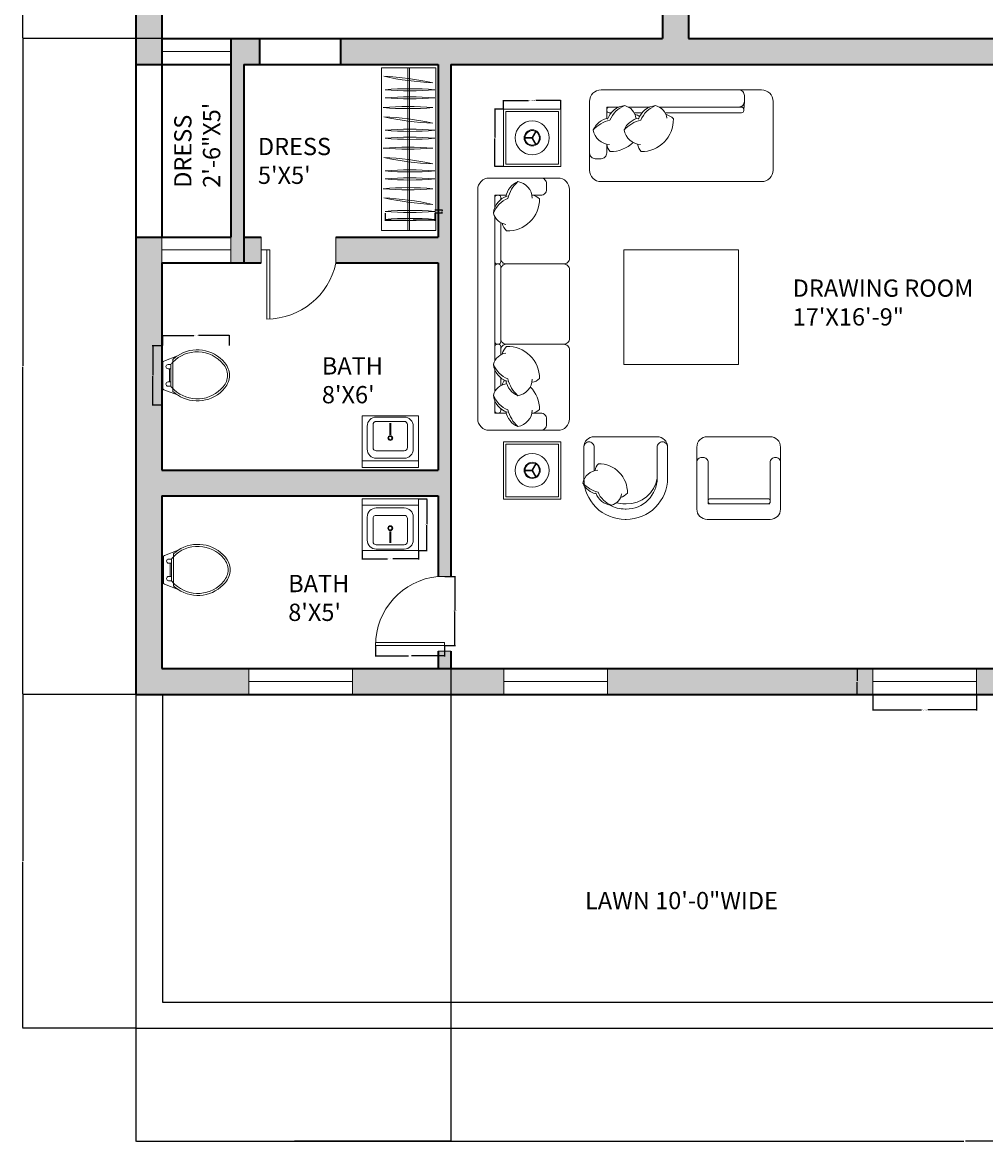
# Model space of a CAD drawing. Units: inches. Extents: x -9 to 646, y -802 to 47.
# Tile 1 of 17: x -9 to 326, y -802 to -412. Entities that reach past the tile are written whole.
import ezdxf

# ---------------------------------------------------------------- set-up
doc = ezdxf.new("R2010")
doc.units = ezdxf.units.IN
doc.header["$MEASUREMENT"] = 0
for name, color, linetype, lineweight in [('A-ANNO-DIMS', 2, 'Continuous', 18), ('A-AREA-IDEN', 7, 'Continuous', 18), ('A-DOOR', 4, 'Continuous', 18), ('A-FLOR-CASE', 8, 'Continuous', 18), ('A-FLOR-FIXT', 9, 'Continuous', 18), ('A-FURN', 8, 'Continuous', 15), ('A-GLAZ', 4, 'Continuous', 15), ('A-WALL', 7, 'Continuous', 35), ('A-WALL-PATT', 5, 'Continuous', 9), ('C-SITE', 7, 'Continuous', 25)]:
    doc.layers.add(name, color=color, linetype=linetype, lineweight=lineweight)
doc.styles.get("Standard").update_dxf_attribs({"font": 'arial.ttf'})
doc.dimstyles.get("Standard").update_dxf_attribs({"dimtxt": 0.18, "dimasz": 0.18, "dimexe": 0.18, "dimexo": 0.0625, "dimgap": 0.09, "dimtad": 0, "dimtih": 1, "dimtoh": 1, "dimdec": 0, "dimzin": 0, "dimdsep": 46, "dimlunit": 3, "dimtxsty": 'Standard', "dimcen": 0.09, "dimadec": 0, "dimazin": 0, "dimtfac": 1, "dimtdec": 0, "dimtofl": 0, "dimtmove": 0, "dimatfit": 3, "dimfxl": 1, "dimtolj": 1, "dimtzin": 0, "dimarcsym": 0})

# ---------------------------------------------------------------- blocks, each defined once
blk = doc.blocks.new('М14 600х655')
for p, q in [((-655, 600), (-655, 0)), ((-655, 600), (-655, 0)), ((-655, 0), (-655, 600)), ((0, 600), (-655, 600)), ((0, 525), (-655, 525)), ((0, 0), (0, 600)), ((-165, 494), (-490, 494)), ((-165, 408), (-490, 408)), ((-596, 388), (-596, 121)), ((-528, 370), (-528, 103)), ((-127, 103), (-127, 370)), ((-59, 121), (-59, 388)), ((-334, 87), (-334, 220)), ((-321, 87), (-321, 220)), ((-655, 0), (-655, 0)), ((-655, 0), (-655, 0)), ((-655, 0), (0, 0)), ((-655, 0), (0, 0)), ((-490, 65), (-165, 65)), ((-490, 15), (-165, 15))]:
    blk.add_line(p, q)
for radius in [27.6, 19.3]:
    blk.add_circle((-327, 259), radius)
for centre, radius, start, end in [((-490, 388), 106, 90, 180), ((-490, 370), 38.2, 90, 180), ((-165, 388), 106, 0, 90), ((-165, 370), 38.2, 0, 90), ((-490, 121), 106, 180, 270), ((-490, 103), 38.2, 180, 270), ((-165, 121), 106, 270, 0), ((-165, 103), 38.2, 270, 0)]:
    blk.add_arc(centre, radius, start, end)
blk = doc.blocks.new('WATER-CLOSET')
for p, q in [((3.52, 13.45), (3.52, 14.43)), ((3.52, 13.45), (3.52, 8.88)), ((3.52, 4.31), (3.52, 8.88)), ((3.52, 3.33), (3.52, 4.31))]:
    blk.add_line(p, q)
for points in [[(0, 8.88), (0, 13.32, -0.31031), (0.37, 13.86), (5.11, 15.69, -0.209071)], [(3.52, 13.45, -0.448546), (21.03, 12.81, -0.162618), (22.55, 8.88, -0.470877)], [(3.52, 14.43, -0.040937), (5.11, 15.69, -0.163732)], [(5.11, 15.69, -0.383919), (21.57, 13.25, -0.163732), (23.24, 8.88, -0.359733)], [(2.82, 12.65), (1.84, 12.65, 1), (1.84, 11.17), (2.35, 11.17)], [(2.82, 12.65, -0.022712), (3.52, 13.45, -0.162618)], [(2.82, 8.88), (2.82, 12.65, -0.476108)], [(0, 8.88), (0, 4.44, 0.31031), (0.37, 3.9), (5.11, 2.07, 0.209071)], [(2.82, 8.88), (2.82, 5.11, 0.022712)], [(3.99, 3.84, 0.431639), (21.03, 4.95, 0.162618), (22.55, 8.88, 0.470877)], [(5.11, 2.07, 0.383919), (21.57, 4.51, 0.163732), (23.24, 8.88, 0.359733)], [(2.82, 5.11), (1.84, 5.11, -1), (1.84, 6.59), (2.35, 6.59)], [(2.82, 5.11, 0.022712), (3.52, 4.31, 0.162618)], [(3.52, 4.31, 0.014165), (3.99, 3.84, 0.162618)], [(3.52, 3.33, 0.040937), (5.11, 2.07, 0.163732)]]:
    blk.add_lwpolyline(points, format="xyb")
for points in [[(2.35, 11.17), (2.35, 6.59)], [(2.35, 11.17), (2.82, 11.17)], [(2.35, 6.59), (2.82, 6.59)]]:
    blk.add_lwpolyline(points)
blk = doc.blocks.new('END-TABLE-SQUARE')
for p, q in [((9.86, 10.03), (11.26, 12.46)), ((10.07, 9.9), (11.48, 12.34)), ((9.96, 10.09), (7.15, 10.09)), ((9.96, 9.84), (7.15, 9.84)), ((9.86, 9.9), (11.26, 7.47)), ((10.07, 10.03), (11.48, 7.59))]:
    blk.add_line(p, q)
at = {"ltscale": 0.03}
blk.add_lwpolyline([(19.93, 19.93), (19.93, 0), (0, 0), (0, 19.93)], close=True, dxfattribs=at)
blk.add_lwpolyline([(19.13, 0.8), (19.13, 19.13), (0.8, 19.13), (0.8, 0.8)], close=True)
for radius in [5.88, 2.81, 2.52]:
    blk.add_circle((9.96, 9.97), radius)
blk = doc.blocks.new('CLOSET-GARMENT-SHORT')
for centre, start, end in [((8.63, -98.34), 85.0028, 94.9972), ((8.63, -98.34), 85.0028, 94.9972), ((8.63, 99.1), 265.0028, 274.9972), ((8.63, 99.1), 265.0028, 274.9972)]:
    blk.add_arc(centre, 99.09, start, end)
blk = doc.blocks.new('DOOR-LEAF-24-WALL9')
for p, q in [((0, 0), (0, 24)), ((1, 0), (1, 24)), ((0, 0), (1, 0))]:
    blk.add_line(p, q)
blk.add_arc((0, -0.52), 24.52, 11.8123, 90)
blk = doc.blocks.new('DOOR-LEAF-24-WALL4_5')
for p, q in [((0, 24), (24, 24)), ((0, 24), (0, 23)), ((0, 23), (24, 23))]:
    blk.add_line(p, q)
blk.add_arc((-0.11, 24), 24.12, 275.6311, 0)
blk = doc.blocks.new('GLAZING-36')
for p, q in [((0, 36), (0, 0)), ((4.5, 36), (4.5, 0)), ((9, 0), (9, 36))]:
    blk.add_line(p, q)
blk = doc.blocks.new('GLAZING-24')
for p, q in [((0, 9), (24, 9)), ((0, 4.5), (24, 4.5)), ((24, 0), (0, 0))]:
    blk.add_line(p, q)
blk = doc.blocks.new('*D19')
at = {"layer": 'A-ANNO-DIMS', "color": 0, "lineweight": -2, "transparency": 16777216}
for p, q in [((116.94, -478.74), (116.94, -481.44)), ((117.12, -481.26), (124.38, -481.26)), ((134.02, -481.26), (126.76, -481.26)), ((134.2, -478.74), (134.2, -481.44))]:
    blk.add_line(p, q, dxfattribs=at)
at = {"layer": 'A-ANNO-DIMS', "color": 0, "transparency": 16777216}
for points in [[(117.12, -481.23), (117.12, -481.29), (116.94, -481.26)], [(134.02, -481.23), (134.02, -481.29), (134.2, -481.26)]]:
    blk.add_solid(points, dxfattribs=at)
at = {"layer": 'Defpoints', "color": 0, "transparency": 16777216}
for p in [(116.94, -478.67), (134.2, -478.67), (134.2, -481.26)]:
    blk.add_point(p, dxfattribs=at)
at = {"layer": 'A-ANNO-DIMS', "color": 0, "transparency": 16777216, "insert": (125.57, -481.26), "char_height": 0.18, "attachment_point": 5}
blk.add_mtext('\\A1;GARMENT 17 TYP.', dxfattribs=at)
blk = doc.blocks.new('*D20')
at = {"layer": 'A-ANNO-DIMS', "color": 0, "lineweight": -2, "transparency": 16777216}
for p, q in [((134.26, -477.67), (136.97, -477.67)), ((136.79, -477.85), (136.79, -477.99)), ((136.79, -478.49), (136.79, -478.35)), ((134.26, -478.67), (136.97, -478.67))]:
    blk.add_line(p, q, dxfattribs=at)
at = {"layer": 'A-ANNO-DIMS', "color": 0, "transparency": 16777216}
for points in [[(136.76, -477.85), (136.82, -477.85), (136.79, -477.67)], [(136.76, -478.49), (136.82, -478.49), (136.79, -478.67)]]:
    blk.add_solid(points, dxfattribs=at)
at = {"layer": 'Defpoints', "color": 0, "transparency": 16777216}
for p in [(134.2, -477.67), (136.79, -477.67), (134.2, -478.67)]:
    blk.add_point(p, dxfattribs=at)
at = {"layer": 'A-ANNO-DIMS', "color": 0, "transparency": 16777216, "insert": (136.79, -478.17), "char_height": 0.18, "attachment_point": 5}
blk.add_mtext('\\A1;1 TYP.', dxfattribs=at)
blk = doc.blocks.new('*D23')
at = {"layer": 'A-ANNO-DIMS', "color": 0, "lineweight": -2, "transparency": 16777216}
for p, q in [((137.69, -605.07), (141.4, -605.07)), ((141.22, -605.25), (141.22, -616.89)), ((141.22, -628.89), (141.22, -617.25)), ((137.69, -629.07), (141.4, -629.07))]:
    blk.add_line(p, q, dxfattribs=at)
at = {"layer": 'A-ANNO-DIMS', "color": 0, "transparency": 16777216}
for points in [[(141.19, -605.25), (141.25, -605.25), (141.22, -605.07)], [(141.19, -628.89), (141.25, -628.89), (141.22, -629.07)]]:
    blk.add_solid(points, dxfattribs=at)
at = {"layer": 'Defpoints', "color": 0, "transparency": 16777216}
for p in [(137.62, -605.07), (137.62, -629.07), (141.22, -629.07)]:
    blk.add_point(p, dxfattribs=at)
at = {"layer": 'A-ANNO-DIMS', "color": 0, "transparency": 16777216, "insert": (141.22, -617.07), "char_height": 0.18, "attachment_point": 5}
blk.add_mtext('\\A1;DOOR 24 TYP.', dxfattribs=at)
blk = doc.blocks.new('*D24')
at = {"layer": 'A-ANNO-DIMS', "color": 0, "lineweight": -2, "transparency": 16777216}
for p, q in [((113.62, -629.13), (113.62, -632.85)), ((137.62, -629.13), (137.62, -632.85)), ((113.8, -632.67), (125.09, -632.67)), ((137.44, -632.67), (126.15, -632.67))]:
    blk.add_line(p, q, dxfattribs=at)
at = {"layer": 'A-ANNO-DIMS', "color": 0, "transparency": 16777216}
for points in [[(113.8, -632.64), (113.8, -632.7), (113.62, -632.67)], [(137.44, -632.64), (137.44, -632.7), (137.62, -632.67)]]:
    blk.add_solid(points, dxfattribs=at)
at = {"layer": 'Defpoints', "color": 0, "transparency": 16777216}
for p in [(113.62, -629.07), (137.62, -629.07), (113.62, -632.67)]:
    blk.add_point(p, dxfattribs=at)
at = {"layer": 'A-ANNO-DIMS', "color": 0, "transparency": 16777216, "insert": (125.62, -632.67), "char_height": 0.18, "attachment_point": 5}
blk.add_mtext('\\A1;24 TYP.', dxfattribs=at)
blk = doc.blocks.new('*D27')
at = {"layer": 'A-ANNO-DIMS', "color": 0, "lineweight": -2, "transparency": 16777216}
for p, q in [((286.47, -646.13), (286.47, -651.65)), ((322.47, -646.13), (322.47, -651.65)), ((286.65, -651.47), (303.35, -651.47)), ((322.29, -651.47), (305.59, -651.47))]:
    blk.add_line(p, q, dxfattribs=at)
at = {"layer": 'A-ANNO-DIMS', "color": 0, "transparency": 16777216}
for points in [[(286.65, -651.44), (286.65, -651.5), (286.47, -651.47)], [(322.29, -651.44), (322.29, -651.5), (322.47, -651.47)]]:
    blk.add_solid(points, dxfattribs=at)
at = {"layer": 'Defpoints', "color": 0, "transparency": 16777216}
for p in [(286.47, -646.07), (322.47, -646.07), (286.47, -651.47)]:
    blk.add_point(p, dxfattribs=at)
at = {"layer": 'A-ANNO-DIMS', "color": 0, "transparency": 16777216, "insert": (304.47, -651.47), "char_height": 0.18, "attachment_point": 5}
blk.add_mtext('\\A1;WINDOW 36 TYP.', dxfattribs=at)
blk = doc.blocks.new('*D28')
at = {"layer": 'A-ANNO-DIMS', "color": 0, "lineweight": -2, "transparency": 16777216}
for p, q in [((286.41, -637.07), (280.89, -637.07)), ((281.07, -637.25), (281.07, -641.39)), ((281.07, -645.89), (281.07, -641.75)), ((286.41, -646.07), (280.89, -646.07))]:
    blk.add_line(p, q, dxfattribs=at)
at = {"layer": 'A-ANNO-DIMS', "color": 0, "transparency": 16777216}
for points in [[(281.04, -637.25), (281.1, -637.25), (281.07, -637.07)], [(281.04, -645.89), (281.1, -645.89), (281.07, -646.07)]]:
    blk.add_solid(points, dxfattribs=at)
at = {"layer": 'Defpoints', "color": 0, "transparency": 16777216}
for p in [(281.07, -637.07), (286.47, -637.07), (286.47, -646.07)]:
    blk.add_point(p, dxfattribs=at)
at = {"layer": 'A-ANNO-DIMS', "color": 0, "transparency": 16777216, "insert": (281.07, -641.57), "char_height": 0.18, "attachment_point": 5}
blk.add_mtext('\\A1;9 TYP.', dxfattribs=at)
blk = doc.blocks.new('*D31')
at = {"layer": 'A-ANNO-DIMS', "color": 0, "lineweight": -2, "transparency": 16777216}
for p, q in [((108.99, -596.07), (108.99, -599.12)), ((109.17, -598.94), (117.83, -598.94)), ((128.36, -598.94), (119.7, -598.94)), ((128.54, -596.07), (128.54, -599.12))]:
    blk.add_line(p, q, dxfattribs=at)
at = {"layer": 'A-ANNO-DIMS', "color": 0, "transparency": 16777216}
for points in [[(109.17, -598.91), (109.17, -598.97), (108.99, -598.94)], [(128.36, -598.91), (128.36, -598.97), (128.54, -598.94)]]:
    blk.add_solid(points, dxfattribs=at)
at = {"layer": 'Defpoints', "color": 0, "transparency": 16777216}
for p in [(108.99, -596), (128.54, -596), (128.54, -598.94)]:
    blk.add_point(p, dxfattribs=at)
at = {"layer": 'A-ANNO-DIMS', "color": 0, "transparency": 16777216, "insert": (118.76, -598.94), "char_height": 0.18, "attachment_point": 5}
blk.add_mtext('\\A1;BASIN 20 TYP.', dxfattribs=at)
blk = doc.blocks.new('*D32')
at = {"layer": 'A-ANNO-DIMS', "color": 0, "lineweight": -2, "transparency": 16777216}
for p, q in [((128.6, -578.1), (131.65, -578.1)), ((131.47, -578.28), (131.47, -586.87)), ((131.47, -595.82), (131.47, -587.23)), ((128.6, -596), (131.65, -596))]:
    blk.add_line(p, q, dxfattribs=at)
at = {"layer": 'A-ANNO-DIMS', "color": 0, "transparency": 16777216}
for points in [[(131.44, -578.28), (131.5, -578.28), (131.47, -578.1)], [(131.44, -595.82), (131.5, -595.82), (131.47, -596)]]:
    blk.add_solid(points, dxfattribs=at)
at = {"layer": 'Defpoints', "color": 0, "transparency": 16777216}
for p in [(128.54, -578.1), (131.47, -578.1), (128.54, -596)]:
    blk.add_point(p, dxfattribs=at)
at = {"layer": 'A-ANNO-DIMS', "color": 0, "transparency": 16777216, "insert": (131.47, -587.05), "char_height": 0.18, "attachment_point": 5}
blk.add_mtext('\\A1;18 TYP.', dxfattribs=at)
blk = doc.blocks.new('*D33')
at = {"layer": 'A-ANNO-DIMS', "color": 0, "lineweight": -2, "transparency": 16777216}
for p, q in [((39.69, -524.77), (39.69, -521.17)), ((62.93, -524.77), (62.93, -521.17)), ((39.87, -521.35), (50.54, -521.35)), ((62.75, -521.35), (52.09, -521.35))]:
    blk.add_line(p, q, dxfattribs=at)
at = {"layer": 'A-ANNO-DIMS', "color": 0, "transparency": 16777216}
for points in [[(39.87, -521.32), (39.87, -521.38), (39.69, -521.35)], [(62.75, -521.32), (62.75, -521.38), (62.93, -521.35)]]:
    blk.add_solid(points, dxfattribs=at)
at = {"layer": 'Defpoints', "color": 0, "transparency": 16777216}
for p in [(39.69, -524.84), (62.93, -521.35), (62.93, -524.84)]:
    blk.add_point(p, dxfattribs=at)
at = {"layer": 'A-ANNO-DIMS', "color": 0, "transparency": 16777216, "insert": (51.31, -521.35), "char_height": 0.18, "attachment_point": 5}
blk.add_mtext('\\A1;WC 23 TYP.', dxfattribs=at)
blk = doc.blocks.new('*D34')
at = {"layer": 'A-ANNO-DIMS', "color": 0, "lineweight": -2, "transparency": 16777216}
for p, q in [((39.63, -524.84), (36.02, -524.84)), ((36.2, -525.02), (36.2, -534.98)), ((36.2, -545.31), (36.2, -535.34)), ((39.63, -545.49), (36.02, -545.49))]:
    blk.add_line(p, q, dxfattribs=at)
at = {"layer": 'A-ANNO-DIMS', "color": 0, "transparency": 16777216}
for points in [[(36.17, -525.02), (36.23, -525.02), (36.2, -524.84)], [(36.17, -545.31), (36.23, -545.31), (36.2, -545.49)]]:
    blk.add_solid(points, dxfattribs=at)
at = {"layer": 'Defpoints', "color": 0, "transparency": 16777216}
for p in [(36.2, -524.84), (39.69, -524.84), (39.69, -545.49)]:
    blk.add_point(p, dxfattribs=at)
at = {"layer": 'A-ANNO-DIMS', "color": 0, "transparency": 16777216, "insert": (36.2, -535.16), "char_height": 0.18, "attachment_point": 5}
blk.add_mtext('\\A1;21 TYP.', dxfattribs=at)
blk = doc.blocks.new('*D39')
at = {"layer": 'A-ANNO-DIMS', "color": 0, "lineweight": -2, "transparency": 16777216}
for p, q in [((158.14, -442.59), (158.14, -439.48)), ((178.07, -442.59), (178.07, -439.48)), ((158.32, -439.66), (166.81, -439.66)), ((177.89, -439.66), (169.39, -439.66))]:
    blk.add_line(p, q, dxfattribs=at)
at = {"layer": 'A-ANNO-DIMS', "color": 0, "transparency": 16777216}
for points in [[(158.32, -439.63), (158.32, -439.69), (158.14, -439.66)], [(177.89, -439.63), (177.89, -439.69), (178.07, -439.66)]]:
    blk.add_solid(points, dxfattribs=at)
at = {"layer": 'Defpoints', "color": 0, "transparency": 16777216}
for p in [(158.14, -442.65), (178.07, -439.66), (178.07, -442.65)]:
    blk.add_point(p, dxfattribs=at)
at = {"layer": 'A-ANNO-DIMS', "color": 0, "transparency": 16777216, "insert": (168.1, -439.66), "char_height": 0.18, "attachment_point": 5}
blk.add_mtext('\\A1;SIDE TABLE 20 TYP.', dxfattribs=at)
blk = doc.blocks.new('*D40')
at = {"layer": 'A-ANNO-DIMS', "color": 0, "lineweight": -2, "transparency": 16777216}
for p, q in [((158.08, -442.65), (154.97, -442.65)), ((155.15, -442.83), (155.15, -452.43)), ((155.15, -462.4), (155.15, -452.8)), ((158.08, -462.58), (154.97, -462.58))]:
    blk.add_line(p, q, dxfattribs=at)
at = {"layer": 'A-ANNO-DIMS', "color": 0, "transparency": 16777216}
for points in [[(155.12, -442.83), (155.18, -442.83), (155.15, -442.65)], [(155.12, -462.4), (155.18, -462.4), (155.15, -462.58)]]:
    blk.add_solid(points, dxfattribs=at)
at = {"layer": 'Defpoints', "color": 0, "transparency": 16777216}
for p in [(155.15, -442.65), (158.14, -442.65), (158.14, -462.58)]:
    blk.add_point(p, dxfattribs=at)
at = {"layer": 'A-ANNO-DIMS', "color": 0, "transparency": 16777216, "insert": (155.15, -452.61), "char_height": 0.18, "attachment_point": 5}
blk.add_mtext('\\A1;20 TYP.', dxfattribs=at)
blk = doc.blocks.new('*D49')
at = {"layer": 'A-ANNO-DIMS', "color": 0, "lineweight": -2, "transparency": 16777216}
for p, q in [((30.37, -762.13), (30.37, -801.5)), ((606.37, -762.13), (606.37, -801.5)), ((30.55, -801.32), (318.08, -801.32)), ((606.19, -801.32), (318.66, -801.32))]:
    blk.add_line(p, q, dxfattribs=at)
at = {"layer": 'A-ANNO-DIMS', "color": 0, "transparency": 16777216}
for points in [[(30.55, -801.29), (30.55, -801.35), (30.37, -801.32)], [(606.19, -801.29), (606.19, -801.35), (606.37, -801.32)]]:
    blk.add_solid(points, dxfattribs=at)
at = {"layer": 'Defpoints', "color": 0, "transparency": 16777216}
for p in [(30.37, -762.07), (606.37, -762.07), (606.37, -801.32)]:
    blk.add_point(p, dxfattribs=at)
at = {"layer": 'A-ANNO-DIMS', "color": 0, "transparency": 16777216, "insert": (318.37, -801.32), "char_height": 0.18, "attachment_point": 5}
blk.add_mtext('\\A1;576', dxfattribs=at)
blk = doc.blocks.new('*D55')
at = {"layer": 'A-ANNO-DIMS', "color": 0, "lineweight": -2, "transparency": 16777216}
for p, q in [((39.31, -253.07), (-9.06, -253.07)), ((-8.88, -253.25), (-8.88, -335.39)), ((-8.88, -417.89), (-8.88, -335.75)), ((39.31, -418.07), (-9.06, -418.07))]:
    blk.add_line(p, q, dxfattribs=at)
at = {"layer": 'A-ANNO-DIMS', "color": 0, "transparency": 16777216}
for points in [[(-8.91, -253.25), (-8.85, -253.25), (-8.88, -253.07)], [(-8.91, -417.89), (-8.85, -417.89), (-8.88, -418.07)]]:
    blk.add_solid(points, dxfattribs=at)
at = {"layer": 'Defpoints', "color": 0, "transparency": 16777216}
for p in [(39.37, -253.07), (-8.88, -418.07), (39.37, -418.07)]:
    blk.add_point(p, dxfattribs=at)
at = {"layer": 'A-ANNO-DIMS', "color": 0, "transparency": 16777216, "insert": (-8.88, -335.57), "char_height": 0.18, "attachment_point": 5}
blk.add_mtext('\\A1;165', dxfattribs=at)
blk = doc.blocks.new('*D56')
at = {"layer": 'A-ANNO-DIMS', "color": 0, "lineweight": -2, "transparency": 16777216}
for p, q in [((213.31, -418.07), (-9.06, -418.07)), ((-8.88, -418.25), (-8.88, -531.89)), ((-8.88, -645.89), (-8.88, -532.25)), ((30.31, -646.07), (-9.06, -646.07))]:
    blk.add_line(p, q, dxfattribs=at)
at = {"layer": 'A-ANNO-DIMS', "color": 0, "transparency": 16777216}
for points in [[(-8.91, -418.25), (-8.85, -418.25), (-8.88, -418.07)], [(-8.91, -645.89), (-8.85, -645.89), (-8.88, -646.07)]]:
    blk.add_solid(points, dxfattribs=at)
at = {"layer": 'Defpoints', "color": 0, "transparency": 16777216}
for p in [(213.37, -418.07), (-8.88, -646.07), (30.37, -646.07)]:
    blk.add_point(p, dxfattribs=at)
at = {"layer": 'A-ANNO-DIMS', "color": 0, "transparency": 16777216, "insert": (-8.88, -532.07), "char_height": 0.18, "attachment_point": 5}
blk.add_mtext('\\A1;228', dxfattribs=at)
blk = doc.blocks.new('*D57')
at = {"layer": 'A-ANNO-DIMS', "color": 0, "lineweight": -2, "transparency": 16777216}
for p, q in [((30.31, -646.07), (-9.06, -646.07)), ((-8.88, -646.25), (-8.88, -703.89)), ((-8.88, -761.89), (-8.88, -704.25)), ((30.31, -762.07), (-9.06, -762.07))]:
    blk.add_line(p, q, dxfattribs=at)
at = {"layer": 'A-ANNO-DIMS', "color": 0, "transparency": 16777216}
for points in [[(-8.91, -646.25), (-8.85, -646.25), (-8.88, -646.07)], [(-8.91, -761.89), (-8.85, -761.89), (-8.88, -762.07)]]:
    blk.add_solid(points, dxfattribs=at)
at = {"layer": 'Defpoints', "color": 0, "transparency": 16777216}
for p in [(30.37, -646.07), (-8.88, -762.07), (30.37, -762.07)]:
    blk.add_point(p, dxfattribs=at)
at = {"layer": 'A-ANNO-DIMS', "color": 0, "transparency": 16777216, "insert": (-8.88, -704.07), "char_height": 0.18, "attachment_point": 5}
blk.add_mtext('\\A1;116', dxfattribs=at)
blk = doc.blocks.new('*D58')
at = {"layer": 'A-ANNO-DIMS', "color": 0, "lineweight": -2, "transparency": 16777216}
for p, q in [((139.87, -637.13), (139.87, -801.5)), ((30.37, -646.13), (30.37, -801.5)), ((30.55, -801.32), (84.74, -801.32)), ((139.69, -801.32), (85.51, -801.32))]:
    blk.add_line(p, q, dxfattribs=at)
at = {"layer": 'A-ANNO-DIMS', "color": 0, "transparency": 16777216}
for points in [[(30.55, -801.29), (30.55, -801.35), (30.37, -801.32)], [(139.69, -801.29), (139.69, -801.35), (139.87, -801.32)]]:
    blk.add_solid(points, dxfattribs=at)
at = {"layer": 'Defpoints', "color": 0, "transparency": 16777216}
for p in [(139.87, -637.07), (30.37, -646.07), (139.87, -801.32)]:
    blk.add_point(p, dxfattribs=at)
at = {"layer": 'A-ANNO-DIMS', "color": 0, "transparency": 16777216, "insert": (85.12, -801.32), "char_height": 0.18, "attachment_point": 5}
blk.add_mtext('\\A1;109.5', dxfattribs=at)

msp = doc.modelspace()

# ---------------------------------------------------------------- hatches: boundary and pattern name
at = {"layer": 'A-WALL-PATT'}
h = msp.add_hatch(color=256, dxfattribs=at)
h.dxf.hatch_style = 1
h.paths.add_polyline_path([(73.4, -418.07), (63.37, -418.07), (63.37, -487.07), (63.35, -496.07), (67.87, -496.07), (67.87, -427.07), (73.4, -427.07)])
h.paths.add_polyline_path([(73.87, -487.07), (67.87, -487.07), (67.87, -496.07), (73.87, -496.07)])
h.paths.add_polyline_path([(39.37, -496.07), (39.35, -496.07), (39.35, -487.07), (30.37, -487.07), (30.37, -646.07), (69.62, -646.07), (69.62, -637.07), (39.37, -637.07)])
h.paths.add_polyline_path([(158.27, -637.07), (105.62, -637.07), (105.62, -646.07), (158.27, -646.07)])
h.paths.add_polyline_path([(286.47, -637.07), (194.27, -637.07), (194.27, -646.07), (286.47, -646.07)])
h.paths.add_polyline_path([(357.37, -552.07), (352.87, -552.07), (348.37, -552.07), (348.37, -637.07), (322.47, -637.07), (322.47, -646.07), (357.37, -646.07)])
h.paths.add_polyline_path([(357.37, -459.07), (352.87, -459.07), (348.37, -459.07), (348.37, -526.07), (357.37, -526.07), (357.37, -520.07), (363.37, -520.07), (363.37, -511.07), (357.37, -511.07)], flags=17)
h.paths.add_polyline_path([(39.37, -262.07), (213.37, -262.07), (213.37, -268.07), (222.37, -268.07), (222.37, -247.07), (213.37, -247.07), (213.37, -253.07), (39.37, -253.07), (39.37, -1.07), (222.37, -1.07), (222.37, 7.93), (30.37, 7.93), (30.37, -427.07), (39.36, -427.07), (39.36, -418.07)])
h.paths.add_polyline_path([(570.37, -149.32), (561.37, -149.32), (561.37, -161.07), (433.37, -161.07), (433.37, -165.57), (433.37, -170.07), (438.37, -170.07), (438.37, -176.07), (447.37, -176.07), (447.37, -170.07), (561.37, -170.07), (561.37, -229.57), (570.37, -229.57)])
h.paths.add_polyline_path([(570.37, -289.57), (561.37, -289.57), (561.37, -349.07), (479.37, -349.07), (479.37, -353.57), (479.37, -358.07), (561.37, -358.07), (561.37, -418.07), (447.37, -418.07), (447.37, -358.07), (453.37, -358.07), (453.37, -349.07), (447.37, -349.07), (447.37, -202.07), (442.87, -202.07), (438.37, -202.07), (438.37, -427.07), (561.37, -427.07), (561.37, -451.07), (570.37, -451.07)])
h.paths.add_polyline_path([(570.37, -496.07), (570.37, -487.07), (561.37, -487.07), (561.37, -511.07), (411.37, -511.07), (411.37, -515.57), (411.37, -520.07), (570.37, -520.07)])
h = msp.add_hatch(color=256, dxfattribs=at)
h.dxf.hatch_style = 1
h.paths.add_polyline_path([(363.37, -418.07), (222.37, -418.07), (222.37, -294.07), (217.87, -294.07), (213.37, -294.07), (213.37, -418.07), (101.62, -418.07), (101.62, -427.07), (135.37, -427.07), (135.37, -487.07), (99.87, -487.07), (99.87, -491.57), (99.87, -496.07), (135.37, -496.07), (135.37, -568.07), (39.37, -568.07), (39.37, -496.07), (39.35, -496.07), (39.35, -487.07), (30.37, -487.07), (30.37, -646.07), (69.62, -646.07), (69.62, -637.07), (39.37, -637.07), (39.37, -577.07), (135.37, -577.07), (135.37, -605.07), (137.62, -605.07), (139.87, -605.07), (139.87, -427.07), (348.37, -427.07), (348.37, -433.07), (357.37, -433.07), (357.37, -427.07), (363.37, -427.07)])
h = msp.add_hatch(color=256, dxfattribs=at)
h.dxf.hatch_style = 1
h.paths.add_polyline_path([(139.87, -631.07), (135.37, -631.07), (135.37, -637.07), (139.87, -637.07)])

# ---------------------------------------------------------------- linework, layer by layer
at = {"layer": 'A-DOOR'}
for p, q in [((73.87, -496.07), (73.87, -487.07)), ((99.87, -491.57), (99.87, -487.07)), ((73.87, -491.57), (75.87, -491.57)), ((99.87, -491.57), (99.87, -496.07)), ((137.62, -605.07), (135.37, -605.07)), ((137.62, -605.07), (139.87, -605.07)), ((137.62, -631.07), (137.62, -629.07)), ((139.87, -631.07), (135.37, -631.07))]:
    msp.add_line(p, q, dxfattribs=at)
at = {"layer": 'A-FLOR-CASE'}
for p, q in [((115.77, -428.3), (115.77, -484.79)), ((115.77, -428.3), (134.61, -428.3)), ((115.77, -428.3), (115.77, -484.79)), ((115.77, -428.3), (134.61, -428.3)), ((124.88, -428.3), (124.88, -484.79)), ((124.88, -428.3), (124.88, -484.79)), ((125.5, -428.3), (125.5, -484.79)), ((125.5, -428.3), (125.5, -484.79)), ((134.61, -428.3), (134.61, -484.79)), ((134.61, -428.3), (134.61, -484.79)), ((115.77, -484.79), (134.61, -484.79))]:
    msp.add_line(p, q, dxfattribs=at)
at = {"layer": 'A-FURN'}
msp.add_line((241.83, -439.92), (241.64, -442.91), dxfattribs=at)
at = {"layer": 'A-FURN', "ltscale": 0.03}
for points in [[(251.8, -463.83, -0.414214), (247.81, -467.81), (247.81, -467.81, 0.317837), (247.81, -467.81, -0.414214), (247.81, -467.81), (247.81, -467.81, 1.186185), (247.81, -467.81, -0.414214), (247.81, -467.81), (192.02, -467.81, -0.414214), (188.03, -463.83), (188.03, -439.92, -0.414214), (192.02, -435.93), (247.81, -435.93, -0.414214), (251.8, -439.92)], [(177.07, -466.56, -0.414214), (181.06, -470.55), (181.06, -494.46, -0.414214), (179.06, -496.45, -0.414214), (181.06, -498.45), (181.06, -522.36, -0.414214), (179.06, -524.35, -0.414214), (181.06, -526.34), (181.06, -550.26, -0.414214), (177.07, -554.24), (153.16, -554.24, -0.414214), (149.17, -550.26), (149.17, -470.55, -0.414214), (153.16, -466.56)], [(250.81, -585.22), (250.81, -585.22, 0.414214), (254.4, -581.63), (254.4, -560.07, 0.414214), (250.81, -556.48), (250.81, -556.48), (228.89, -556.48, 0.414214), (225.3, -560.07), (225.3, -581.63, 0.414214), (228.89, -585.22)]]:
    msp.add_lwpolyline(points, format="xyb", close=True, dxfattribs=at)
at = {"layer": 'A-FURN'}
for points in [[(236.75, -441.91), (239.84, -441.91, 0.414214), (241.83, -439.92), (241.83, -437.92, 0.414214), (239.84, -435.93)], [(189.3, -449.86, -0.14773), (195.12, -446.44, -0.213343), (200.26, -441.41, -0.178662)], [(195.53, -443.9), (194.81, -443.9, -0.414214), (194.01, -443.11), (194.01, -442.71, -0.414214), (194.81, -441.91)], [(198.2, -441.91), (194.01, -441.91), (194.01, -445.83, -0.414214)], [(194.32, -446.16, -0.306663), (200.26, -441.41, -0.30633), (204.14, -445.75, 0.872847)], [(194.81, -441.91), (198.2, -441.91, -0.414214)], [(200.03, -449.86, -0.14773), (205.86, -446.44, -0.213343), (211, -441.41, -0.178662)], [(201.52, -441.91), (208.94, -441.91, -0.414214)], [(205.05, -446.16, -0.306663), (211, -441.41, -0.30633), (214.88, -445.75, 0.872847)], [(212.25, -441.91), (240.84, -441.91, -0.414214), (241.64, -442.71), (241.64, -443.11, -0.414214), (240.84, -443.9), (214.26, -443.9, -0.414214)], [(195.01, -454.88, -0.356772), (189.3, -449.86, -0.249542), (194.47, -445.72, 9.61688)], [(205.74, -454.88, -0.356772), (200.03, -449.86, -0.249542), (205.21, -445.72, 9.61688)], [(206.26, -443.9), (203.52, -443.9, -0.414214)], [(205.44, -445.19, 0.071865), (203.77, -444.41, -7.115464)], [(204.74, -454.76, 0.165541), (205.97, -457.4, 0.425989), (217.16, -445.98, 0.121523), (214.51, -444.41, -7.115464)], [(194.01, -454.76), (194.01, -457.85, -0.414214), (192.02, -459.84), (190.02, -459.84, -0.414214), (188.03, -457.85)], [(194, -454.76, 0.165541), (195.24, -457.4, 0.200231), (203.15, -454.19, 0.121523)], [(171.09, -466.56, -0.414214), (173.09, -468.56), (173.09, -470.55, -0.414214), (171.09, -472.54), (168.01, -472.54)], [(163.1, -467.83, 0.14773), (159.68, -473.66, 0.213343), (154.66, -478.79)], [(168.13, -473.54, 0.356772), (163.1, -467.83, 0.249542), (158.96, -473)], [(159.41, -472.85, 0.306663), (154.66, -478.79, 0.30633), (158.99, -482.68)], [(157.14, -474.06), (157.14, -473.34, 0.414214), (156.35, -472.54), (155.95, -472.54, 0.414214), (155.15, -473.34)], [(155.15, -473.34), (155.15, -476.73, 0.412535)], [(168, -472.54, -0.165541), (170.64, -473.77, -0.425989), (159.22, -484.96, -0.121523), (157.65, -482.3)], [(155.15, -480.05), (155.15, -495.66, 0.414214), (155.95, -496.45), (156.35, -496.45, 0.414214), (157.14, -495.66), (157.14, -482.05, 0.412652)], [(157.14, -494.46, 0.414214), (159.14, -496.45), (179.06, -496.45, 0.415249)], [(157.14, -498.45, -0.414214), (159.14, -496.45)], [(155.15, -530.02), (155.15, -525.15, -0.414214), (155.95, -524.35), (156.35, -524.35, -0.414214), (157.14, -525.15), (157.14, -528.01, -0.126313)], [(157.14, -522.36, 0.414214), (159.14, -524.35)], [(157.14, -526.34, -0.414214), (159.14, -524.35), (179.06, -524.35, -0.41732)], [(168, -537.53, 0.165541), (170.64, -536.3, 0.425989), (159.22, -525.11, 0.121523), (157.65, -527.77)], [(159.41, -537.22, -0.306663), (154.66, -531.28, -0.30633), (158.99, -527.39)], [(163.1, -542.24, -0.14773), (159.68, -536.41, -0.213343), (154.66, -531.28)], [(155.15, -540.76), (155.15, -533.34, -0.414747)], [(157.14, -536.01), (157.14, -538.75, -0.414599)], [(158.43, -536.83, 0.071865), (157.65, -538.5)], [(168.13, -536.53, -0.356772), (163.1, -542.24, -0.249542), (158.96, -537.06)], [(159.41, -547.95, -0.306663), (154.66, -542.01, -0.30633), (158.99, -538.13)], [(168, -548.27, 0.165541), (170.64, -547.03, 0.200231), (167.43, -539.12)], [(163.1, -552.97, -0.14773), (159.68, -547.15, -0.213343), (154.66, -542.01)], [(155.15, -544.07), (155.15, -548.26), (159.07, -548.26, -0.414352)], [(155.15, -547.47), (155.15, -544.07, -0.414469)], [(157.14, -546.74), (157.14, -547.47, -0.414214), (156.35, -548.26), (155.95, -548.26, -0.414214), (155.15, -547.47)], [(168.13, -547.26, -0.356772), (163.1, -552.97, -0.249542), (158.96, -547.8)], [(168.01, -548.26), (171.09, -548.26, -0.414214), (173.09, -550.26), (173.09, -552.25, -0.414214), (171.09, -554.24)], [(189.62, -568.33), (189.62, -560.07, 0.414214), (187.83, -558.27), (187.83, -558.27, 0.414214), (186.03, -560.07)], [(211.54, -570.85), (211.54, -560.07, -0.414214), (213.34, -558.27), (213.34, -558.27, -0.414214), (215.14, -560.07)], [(225.3, -565.46, -0.414214), (227.09, -563.66), (227.45, -563.66, -0.414214), (229.25, -565.46), (229.25, -568.24)], [(250.81, -578.75), (250.81, -565.46, -0.414214), (252.61, -563.66), (252.61, -563.66, -0.414214), (254.4, -565.46)], [(189.98, -568.24, -0.165541), (191.09, -565.87, -0.425989), (201.18, -576.16, -0.121523), (198.79, -577.58, 7.115464)], [(190.89, -568.13, 0.356772), (185.74, -572.66, 0.249542), (190.4, -576.39, -9.61688)], [(211.54, -570.85, -0.372719), (200.76, -579.83), (200.58, -579.83)], [(211.54, -570.85, -0.414214), (200.76, -581.63), (200.58, -581.63)], [(185.74, -572.66, 0.14773), (190.99, -575.75, 0.213343), (195.62, -580.28, 0.178662)], [(190.26, -576, 0.306663), (195.62, -580.28, 0.30633), (199.12, -576.37, -0.872847)], [(197.34, -579.45, 0.072384), (200.41, -579.83), (200.58, -579.83)], [(237.83, -578.04), (229.97, -578.04, 0.414214), (229.25, -578.75), (229.25, -579.11, 0.414214), (229.97, -579.83)], [(236.02, -579.83), (250.09, -579.83, 0.414214), (250.81, -579.11), (250.81, -578.75, 0.414214), (250.09, -578.04), (237.83, -578.04, 0.414214)], [(195.05, -580.21, 0.130591), (200.41, -581.63), (200.58, -581.63)], [(229.97, -579.83), (236.02, -579.83, 0.414214)]]:
    msp.add_lwpolyline(points, format="xyb", dxfattribs=at)
for points in [[(208.94, -441.91), (201.52, -441.91)], [(236.75, -441.91), (212.25, -441.91)], [(159.07, -472.54), (155.15, -472.54), (155.15, -476.73)], [(155.15, -480.05), (155.15, -530.02)], [(155.15, -533.34), (155.15, -540.76)], [(229.25, -568.24), (229.25, -579.83), (236.02, -579.83)], [(236.02, -579.83), (250.63, -579.83)]]:
    msp.add_lwpolyline(points, dxfattribs=at)
at = {"layer": 'A-FURN', "ltscale": 0.03}
msp.add_lwpolyline([(239.84, -531.33), (239.84, -491.47), (199.99, -491.47), (199.99, -531.33)], close=True, dxfattribs=at)
at = {"layer": 'A-FURN'}
msp.add_lwpolyline([(155.15, -523.55), (155.15, -497.25, -0.414214), (155.95, -496.45), (156.35, -496.45, -0.414214), (157.14, -497.25), (157.14, -523.55, -0.414214), (156.35, -524.35), (155.95, -524.35, -0.414214)], format="xyb", close=True, dxfattribs=at)
at = {"layer": 'A-FURN', "ltscale": 0.03}
msp.add_lwpolyline([(200.58, -556.48), (211.54, -556.48, -0.414214), (215.14, -560.07), (215.14, -570.85, -0.414214), (200.76, -585.22), (200.58, -585.22), (200.41, -585.22, -0.414214), (186.03, -570.85), (186.03, -560.07, -0.414214), (189.62, -556.48), (200.58, -556.48)], format="xyb", dxfattribs=at)
at = {"layer": 'A-GLAZ'}
for p, q in [((39.36, -427.07), (39.36, -418.07)), ((63.36, -418.07), (63.36, -427.07)), ((63.35, -487.07), (39.35, -487.07)), ((39.35, -487.07), (39.35, -496.07)), ((63.35, -496.07), (63.35, -487.07)), ((39.35, -491.57), (63.35, -491.57)), ((39.35, -496.07), (63.35, -496.07)), ((69.62, -637.07), (69.62, -646.07)), ((105.62, -646.07), (105.62, -637.07)), ((158.27, -637.07), (158.27, -646.07)), ((194.27, -646.07), (194.27, -637.07)), ((286.47, -637.07), (286.47, -646.07)), ((322.47, -646.07), (322.47, -637.07))]:
    msp.add_line(p, q, dxfattribs=at)
at = {"layer": 'A-WALL'}
for p, q in [((30.37, 7.93), (30.37, -646.07)), ((39.37, -262.07), (39.37, -487.07)), ((213.37, -294.07), (213.37, -418.07)), ((222.37, -294.07), (222.37, -418.07)), ((39.37, -418.07), (213.37, -418.07)), ((63.37, -418.07), (63.37, -487.07)), ((73.4, -427.07), (73.4, -418.07)), ((101.62, -427.07), (101.62, -418.07)), ((222.37, -418.07), (438.37, -418.07)), ((30.37, -427.07), (63.37, -427.07)), ((67.87, -427.07), (67.87, -496.07)), ((67.87, -427.07), (135.37, -427.07)), ((135.37, -427.07), (135.37, -487.07)), ((139.87, -427.07), (348.37, -427.07)), ((139.87, -427.07), (139.87, -605.07)), ((30.37, -487.07), (63.37, -487.07)), ((67.87, -487.07), (73.87, -487.07)), ((99.87, -487.07), (135.37, -487.07)), ((39.37, -496.07), (73.87, -496.07)), ((39.37, -496.07), (39.37, -568.07)), ((99.87, -496.07), (135.37, -496.07)), ((135.37, -496.07), (135.37, -568.07)), ((39.37, -568.07), (135.37, -568.07)), ((39.37, -577.07), (135.37, -577.07)), ((39.37, -577.07), (39.37, -637.07)), ((135.37, -577.07), (135.37, -605.07)), ((135.37, -631.07), (135.37, -637.07)), ((139.87, -631.07), (139.87, -637.07)), ((39.37, -637.07), (348.37, -637.07)), ((213.37, -637.07), (222.37, -637.07)), ((213.37, -637.07), (222.37, -637.07)), ((30.37, -646.07), (357.37, -646.07))]:
    msp.add_line(p, q, dxfattribs=at)
at = {"layer": 'C-SITE'}
for p, q in [((30.37, -646.07), (30.37, -762.07)), ((39.59, -646.07), (39.59, -753.07)), ((39.59, -753.07), (348.37, -753.07)), ((30.37, -762.07), (606.37, -762.07))]:
    msp.add_line(p, q, dxfattribs=at)

# ---------------------------------------------------------------- block references
at = {"layer": 'A-DOOR', "extrusion": (0, 0, -1), "zscale": -1, "rotation": 180}
msp.add_blockref('DOOR-LEAF-24-WALL9', (-75.87, -491.57), dxfattribs=at)
at = {"layer": 'A-DOOR', "rotation": 180}
msp.add_blockref('DOOR-LEAF-24-WALL4_5', (137.63, -605.07), dxfattribs=at)
at = {"layer": 'A-FLOR-CASE'}
for p, rotation in [((116.43, -431.58), 352.5051423896663), ((134.2, -435.51), 180), ((133.59, -441.69), 180), ((116.43, -445.65), 352.5051423895279), ((134.2, -449.59), 180), ((133.64, -461.28), 172.505142389491), ((134.2, -466.51), 180), ((133.64, -475.35), 172.505142389491), ((134.2, -480.58), 180)]:
    msp.add_blockref('CLOSET-GARMENT-SHORT', p, dxfattribs=dict(at, rotation=rotation))
for p in [(116.94, -439.06), (116.94, -453.14), (116.33, -456.58), (116.94, -464.48), (116.33, -470.66), (116.94, -478.55)]:
    msp.add_blockref('CLOSET-GARMENT-SHORT', p, dxfattribs=at)
at = {"layer": 'A-FLOR-FIXT'}
for p in [(39.69, -544.04), (39.91, -611.65)]:
    msp.add_blockref('WATER-CLOSET', p, dxfattribs=at)
at = {"layer": 'A-FLOR-FIXT', "xscale": -0.0298457359050645, "yscale": 0.0298457359050645, "zscale": 0.0298457359050645, "rotation": 180}
msp.add_blockref('М14 600х655', (128.54, -549.22), dxfattribs=at)
at = {"layer": 'A-FLOR-FIXT', "xscale": 0.0298457359050645, "yscale": 0.0298457359050645, "zscale": 0.0298457359050645}
msp.add_blockref('М14 600х655', (128.54, -596), dxfattribs=at)
at = {"layer": 'A-FURN'}
msp.add_blockref('END-TABLE-SQUARE', (158.14, -462.58), dxfattribs=at)
at = {"layer": 'A-FURN', "extrusion": (0, 0, -1), "zscale": -1, "rotation": 180}
msp.add_blockref('END-TABLE-SQUARE', (-158.14, -558.22), dxfattribs=at)
at = {"layer": 'A-GLAZ'}
msp.add_blockref('GLAZING-24', (39.36, -427.07), dxfattribs=at)
for p, rotation in [((105.62, -646.07), 90.00000000000036), ((194.27, -646.07), 90.00000000000003), ((322.47, -646.07), 90.00000000000043)]:
    msp.add_blockref('GLAZING-36', p, dxfattribs=dict(at, rotation=rotation))

# ---------------------------------------------------------------- texts
at = {"layer": 'A-AREA-IDEN', "insert": (43.69, -469.97), "char_height": 6, "attachment_point": 1, "rotation": 90}
msp.add_mtext('DRESS\\P2\'-6"X5\'', dxfattribs=at)
at = {"layer": 'A-AREA-IDEN', "char_height": 6, "attachment_point": 1}
for s, insert in [("DRESS\\P5'X5'", (72.78, -452.61)), ('DRAWING ROOM\\P17\'X16\'-9"', (258.62, -501.83)), ("BATH\\P8'X6'", (95, -528.87)), ('LAWN 10\'-0"WIDE', (186.46, -714.71))]:
    msp.add_mtext(s, dxfattribs=dict(at, insert=insert))
at = {"layer": 'A-AREA-IDEN', "insert": (83.31, -604.52), "char_height": 6, "attachment_point": 1}
msp.add_mtext_dynamic_manual_height_columns("BATH\\P8'X5'", width=2.7294, gutter_width=1, heights=[0], dxfattribs=at)

# ---------------------------------------------------------------- dimensions: what is measured, and where the dimension line sits
at = {"layer": 'A-ANNO-DIMS'}
for base, p1, p2, picture, middle in [((-8.88, -418.07), (39.37, -253.07), (39.37, -418.07), '*D55', (-8.88, -335.57)), ((-8.88, -646.07), (213.37, -418.07), (30.37, -646.07), '*D56', (-8.88, -532.07)), ((-8.88, -762.07), (30.37, -646.07), (30.37, -762.07), '*D57', (-8.88, -704.07))]:
    dim = msp.add_linear_dim(base=base, p1=p1, p2=p2, angle=90, dimstyle='Standard', override={"dimdec": 0, "dimlfac": 1, "dimrnd": 0, "dimzin": 0, "dimdsep": 46, "dimlunit": 2}, dxfattribs=at)
    dim.commit()
    dim.dimension.update_dxf_attribs({"geometry": picture, "text_midpoint": middle})
for base, p1, p2, text, picture, middle in [((178.07, -439.66), (158.14, -442.65), (178.07, -442.65), 'SIDE TABLE <> TYP.', '*D39', (168.1, -439.66)), ((134.2, -481.26), (116.94, -478.67), (134.2, -478.67), 'GARMENT <> TYP.', '*D19', (125.57, -481.26)), ((62.93, -521.35), (39.69, -524.84), (62.93, -524.84), 'WC <> TYP.', '*D33', (51.31, -521.35)), ((128.54, -598.94), (108.99, -596), (128.54, -596), 'BASIN <> TYP.', '*D31', (118.76, -598.94))]:
    dim = msp.add_linear_dim(base=base, p1=p1, p2=p2, text=text, dimstyle='Standard', override={"dimdec": 0, "dimlfac": 1, "dimrnd": 0, "dimzin": 0, "dimdsep": 46, "dimlunit": 2}, dxfattribs=at)
    dim.commit()
    dim.dimension.update_dxf_attribs({"geometry": picture, "text_midpoint": middle})
for base, p1, p2, angle, text, picture, middle in [((155.15, -442.65), (158.14, -462.58), (158.14, -442.65), 90, '<> TYP.', '*D40', (155.15, -452.61)), ((136.79, -477.67), (134.2, -478.67), (134.2, -477.67), 90, '<> TYP.', '*D20', (136.79, -478.17)), ((36.2, -524.84), (39.69, -545.49), (39.69, -524.84), 90, '<> TYP.', '*D34', (36.2, -535.16)), ((131.47, -578.1), (128.54, -596), (128.54, -578.1), 90, '<> TYP.', '*D32', (131.47, -587.05)), ((141.22, -629.07), (137.62, -605.07), (137.62, -629.07), 270, 'DOOR <> TYP.', '*D23', (141.22, -617.07)), ((113.62, -632.67), (137.62, -629.07), (113.62, -629.07), 180, '<> TYP.', '*D24', (125.62, -632.67)), ((281.07, -637.07), (286.47, -646.07), (286.47, -637.07), 90, '<> TYP.', '*D28', (281.07, -641.57)), ((286.47, -651.47), (322.47, -646.07), (286.47, -646.07), 180, 'WINDOW <> TYP.', '*D27', (304.47, -651.47))]:
    dim = msp.add_linear_dim(base=base, p1=p1, p2=p2, angle=angle, text=text, dimstyle='Standard', override={"dimdec": 0, "dimlfac": 1, "dimrnd": 0, "dimzin": 0, "dimdsep": 46, "dimlunit": 2}, dxfattribs=at)
    dim.commit()
    dim.dimension.update_dxf_attribs({"geometry": picture, "text_midpoint": middle})
for base, p1, p2, override, picture, middle in [((139.87, -801.32), (30.37, -646.07), (139.87, -637.07), {"dimdec": 1, "dimlfac": 1, "dimrnd": 0, "dimzin": 0, "dimdsep": 46, "dimlunit": 2}, '*D58', (85.12, -801.32)), ((606.37, -801.32), (30.37, -762.07), (606.37, -762.07), {"dimdec": 0, "dimlfac": 1, "dimrnd": 0, "dimzin": 0, "dimdsep": 46, "dimlunit": 2}, '*D49', (318.37, -801.32))]:
    dim = msp.add_linear_dim(base=base, p1=p1, p2=p2, dimstyle='Standard', override=override, dxfattribs=at)
    dim.commit()
    dim.dimension.update_dxf_attribs({"geometry": picture, "text_midpoint": middle})

doc.saveas('drawing.dxf')
